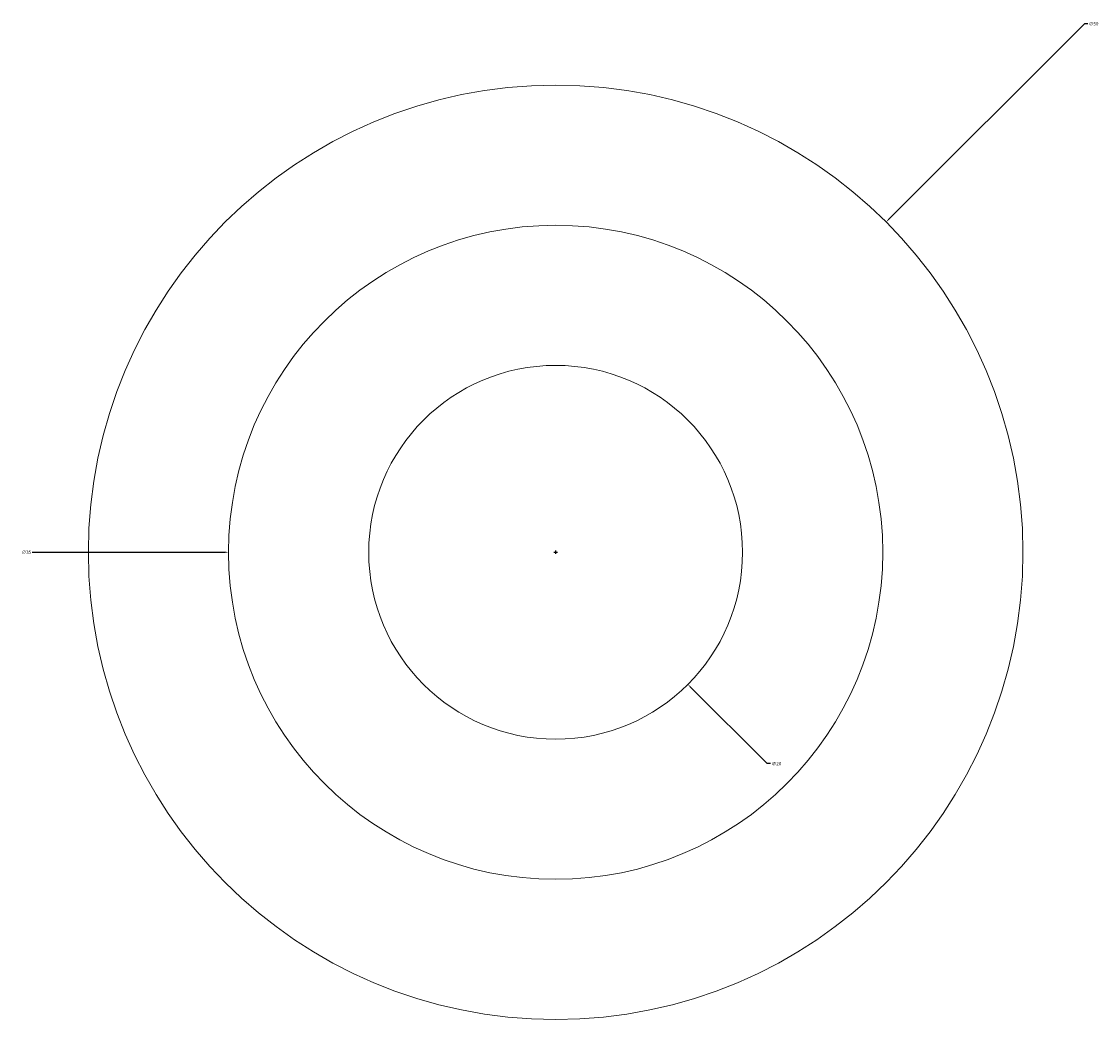
# Model space of a CAD drawing. Units: millimetres. Extents: x 4631 to 4863, y -3 to 1956.
# Tile 2 of 2: x 4631 to 4688, y 1903 to 1956. Entities that reach past the tile are written whole.
import ezdxf

# ---------------------------------------------------------------- set-up
doc = ezdxf.new("R2010")
doc.units = ezdxf.units.MM
doc.layers.add('M-CONS', color=8, linetype='Continuous', lineweight=13)
doc.layers.add('M-DIMS', color=2, linetype='Continuous', lineweight=18)
doc.styles.get("Standard").update_dxf_attribs({"font": 'arial.ttf'})
doc.dimstyles.get("Standard").update_dxf_attribs({"dimtxt": 0.18, "dimasz": 0.18, "dimexe": 0.18, "dimexo": 0.0625, "dimgap": 0.09, "dimtad": 0, "dimtih": 1, "dimtoh": 1, "dimdec": 4, "dimzin": 0, "dimdsep": 46, "dimtxsty": 'Standard', "dimcen": 0.09, "dimadec": 0, "dimazin": 0, "dimtfac": 1, "dimtdec": 4, "dimtofl": 0, "dimtmove": 0, "dimatfit": 3, "dimfxl": 1, "dimtolj": 1, "dimtzin": 0, "dimarcsym": 0})

# ---------------------------------------------------------------- blocks, each defined once
blk = doc.blocks.new('*D4')
at = {"layer": 'Defpoints', "color": 0, "transparency": 16777216}
for p in [(4676.884, 1945.584), (4641.529, 1910.23)]:
    blk.add_point(p, dxfattribs=at)
at = {"layer": 'M-DIMS', "color": 0, "lineweight": -2, "transparency": 16777216}
for p, q in [((4687.491, 1956.191), (4677.012, 1945.712)), ((4687.671, 1956.191), (4687.491, 1956.191)), ((4659.117, 1927.907), (4659.297, 1927.907)), ((4659.207, 1927.817), (4659.207, 1927.997))]:
    blk.add_line(p, q, dxfattribs=at)
at = {"layer": 'M-DIMS', "color": 0, "transparency": 16777216}
blk.add_solid([(4676.991, 1945.733), (4677.033, 1945.691), (4676.884, 1945.584)], dxfattribs=at)
at = {"layer": 'M-DIMS', "color": 0, "transparency": 16777216, "insert": (4687.988, 1956.191), "char_height": 0.18, "attachment_point": 5}
blk.add_mtext('\\A1;∅50', dxfattribs=at)
blk = doc.blocks.new('*D5')
at = {"layer": 'Defpoints', "color": 0, "transparency": 16777216}
for p in [(4641.707, 1927.91), (4676.707, 1927.904)]:
    blk.add_point(p, dxfattribs=at)
at = {"layer": 'M-DIMS', "color": 0, "lineweight": -2, "transparency": 16777216}
for p, q in [((4631.207, 1927.912), (4641.527, 1927.91)), ((4659.117, 1927.907), (4659.297, 1927.907)), ((4659.207, 1927.817), (4659.207, 1927.997))]:
    blk.add_line(p, q, dxfattribs=at)
at = {"layer": 'M-DIMS', "color": 0, "transparency": 16777216}
blk.add_solid([(4641.527, 1927.94), (4641.527, 1927.88), (4641.707, 1927.91)], dxfattribs=at)
at = {"layer": 'M-DIMS', "color": 0, "transparency": 16777216, "insert": (4630.889, 1927.912), "char_height": 0.18, "attachment_point": 5}
blk.add_mtext('\\A1;∅35', dxfattribs=at)
blk = doc.blocks.new('*D6')
at = {"layer": 'Defpoints', "color": 0, "transparency": 16777216}
for p in [(4652.132, 1934.975), (4666.281, 1920.839)]:
    blk.add_point(p, dxfattribs=at)
at = {"layer": 'M-DIMS', "color": 0, "lineweight": -2, "transparency": 16777216}
for p, q in [((4659.117, 1927.907), (4659.297, 1927.907)), ((4659.207, 1927.817), (4659.207, 1927.997)), ((4670.525, 1916.598), (4666.408, 1920.712)), ((4670.705, 1916.598), (4670.525, 1916.598))]:
    blk.add_line(p, q, dxfattribs=at)
at = {"layer": 'M-DIMS', "color": 0, "transparency": 16777216}
blk.add_solid([(4666.429, 1920.733), (4666.387, 1920.691), (4666.281, 1920.839)], dxfattribs=at)
at = {"layer": 'M-DIMS', "color": 0, "transparency": 16777216, "insert": (4671.022, 1916.598), "char_height": 0.18, "attachment_point": 5}
blk.add_mtext('\\A1;∅20', dxfattribs=at)

msp = doc.modelspace()

# ---------------------------------------------------------------- linework, layer by layer
at = {"layer": 'M-CONS'}
msp.add_line((4659.2065, 1902.9071), (4659.2065, 1902.9071, -30), dxfattribs=at)
for radius in [25, 17.5, 10]:
    msp.add_circle((4659.2065, 1927.9071), radius, dxfattribs=at)

# ---------------------------------------------------------------- dimensions: what is measured, and where the dimension line sits
at = {"layer": 'M-DIMS'}
for p1, p2, picture, middle in [((4641.5286, 1910.2297), (4676.8845, 1945.5845), '*D4', (4687.9878, 1956.1909)), ((4652.1323, 1934.975), (4666.2808, 1920.8392), '*D6', (4671.0219, 1916.5985)), ((4676.7065, 1927.9042), (4641.7065, 1927.91), '*D5', (4631.2065, 1927.9117))]:
    dim = msp.add_diameter_dim_2p(p1=p1, p2=p2, dimstyle='Standard', override={"dimdec": 0, "dimlfac": 1, "dimrnd": 0, "dimzin": 0, "dimdsep": 46, "dimlunit": 2}, dxfattribs=at)
    dim.commit()
    dim.dimension.update_dxf_attribs({"geometry": picture, "text_midpoint": middle, "dimtype": 163})

doc.saveas('drawing.dxf')
